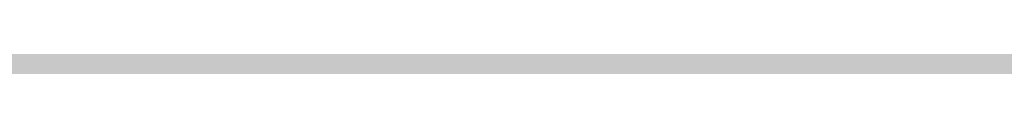
# Model space of a CAD drawing. Units: inches. Extents: x 2091 to 2899, y 967 to 2217.
# Tile 182 of 256: x 2203.16122 to 2203.18039, y 1152.24716 to 1152.24727. Entities that reach past the tile are written whole.
import ezdxf

# ---------------------------------------------------------------- set-up
doc = ezdxf.new("R2010")
doc.units = ezdxf.units.IN
doc.layers.add('A-WALL-PATT', color=141, linetype='Continuous', lineweight=13, true_color=0xadddf7)

msp = doc.modelspace()

# ---------------------------------------------------------------- hatches: boundary and pattern name
at = {"layer": 'A-WALL-PATT'}
h = msp.add_hatch(color=256, dxfattribs=at)
h.dxf.hatch_style = 1
h.paths.add_polyline_path([(2803.143603, 2050.919059), (2203.143603, 2050.919059), (2203.143603, 1090.919059), (2803.143603, 1090.919059)])
h.paths.add_polyline_path([(2635.79885, 1147.540465), (2674.524052, 1147.540465, 0.376086), (2678.529665, 1152.880202), (2678.529665, 1159.556473, 0.333335), (2674.524319, 1163.561846), (2674.524319, 1163.56185), (2674.524319, 1192.93439), (2635.805971, 1192.93439), (2597.087622, 1192.93439), (2597.087622, 1163.561846, 0.333335), (2593.082276, 1159.556473), (2593.082276, 1152.880202, 0.376086), (2597.087889, 1147.540465)], flags=0)
h.paths.add_polyline_path([(2436.010433, 1278.240778, 0.000483), (2435.952643, 1278.215027, -0.001328), (2435.935625, 1278.111693, -0.001711), (2436.11644, 1278.040758, 0.002185)], flags=0)
h.paths.add_polyline_path([(2794.143603, 1143.419059), (2794.143603, 1347.419059), (2543.370171, 1347.419059), (2543.370171, 1351.919059), (2794.143603, 1351.919059), (2794.143603, 1392.713555), (2793.947398, 1392.713555), (2793.947398, 1473.5369), (2794.143603, 1473.5369), (2794.143603, 1531.919059), (2650.143603, 1531.919059), (2650.143603, 1536.419059), (2794.143603, 1536.419059), (2794.143603, 1692.419059), (2609.375609, 1692.419059), (2609.375609, 1644.419059), (2604.875609, 1644.419059), (2604.875609, 1744.919059), (2609.375609, 1744.919059), (2609.375609, 1696.919059), (2794.143603, 1696.919059), (2794.143603, 1780.919059), (2609.643603, 1780.919059), (2493.875609, 1780.919059), (2493.875609, 1785.419059), (2609.643603, 1785.419059), (2794.143603, 1785.419059), (2794.143603, 1847.938821), (2793.951222, 1847.938821), (2793.951222, 1928.762166), (2794.143603, 1928.762166), (2794.143603, 1941.419059), (2614.143603, 1941.419059), (2614.143603, 1821.419059), (2609.643603, 1821.419059), (2609.643603, 1941.419059), (2392.143603, 1941.419059), (2392.143603, 1819.919059), (2387.643603, 1819.919059), (2387.643603, 1941.419059), (2212.143603, 1941.419059), (2212.143603, 1783.919059), (2392.143603, 1783.919059), (2392.143603, 1780.919059), (2212.143603, 1780.919059), (2212.143603, 1629.419059), (2387.643603, 1629.419059), (2387.643603, 1744.919059), (2392.143603, 1744.919059), (2392.143603, 1627.919059), (2317.143603, 1627.919059), (2317.143603, 1551.419059), (2317.143603, 1536.419059), (2459.383591, 1536.419059), (2459.383591, 1602.39648), (2463.883591, 1602.39648), (2463.883591, 1531.919059), (2456.643603, 1531.919059), (2456.643603, 1529.919059), (2452.143603, 1529.919059), (2452.143603, 1531.919059), (2312.643603, 1531.919059), (2312.643603, 1551.419059), (2306.143603, 1551.419059), (2306.143603, 1555.919059), (2308.143603, 1555.919059), (2308.143603, 1551.419059), (2312.643603, 1551.419059), (2312.643603, 1627.919059), (2212.143603, 1627.919059), (2212.143603, 1555.919059), (2270.143603, 1555.919059), (2270.143603, 1551.419059), (2212.143603, 1551.419059), (2212.143603, 1351.919059), (2272.143603, 1351.919059), (2272.143603, 1347.419059), (2212.143603, 1347.419059), (2212.143603, 1275.419059), (2308.143603, 1275.419059), (2308.143603, 1351.919059), (2452.143603, 1351.919059), (2452.143603, 1493.919059), (2456.643603, 1493.919059), (2456.643603, 1347.419059), (2312.643603, 1347.419059), (2312.643603, 1270.919059), (2212.143603, 1270.919059), (2212.143603, 1099.919059), (2281.237523, 1099.919059), (2282.871041, 1110.913803), (2282.008341, 1116.996603), (2278.557741, 1121.420403), (2268.205641, 1128.056203), (2272.087641, 1128.056203), (2273.812941, 1131.927003), (2279.420341, 1134.691903), (2285.027841, 1135.244903), (2287.615841, 1137.456803), (2288.047141, 1138.009803), (2289.341141, 1140.774703), (2291.066541, 1139.668703), (2292.360541, 1135.244903), (2295.379841, 1136.903803), (2296.242541, 1135.797903), (2297.105241, 1133.033003), (2300.124641, 1138.009803), (2303.143941, 1138.009803), (2304.437941, 1135.797903), (2303.143941, 1133.586003), (2306.594641, 1134.691903), (2307.888741, 1133.033003), (2310.908041, 1135.244903), (2313.927441, 1134.138903), (2315.62686, 1132.427102), (2308.320041, 1117.549603), (2290.203841, 1109.807903), (2288.909841, 1103.172103), (2289.272309, 1099.919059), (2434.918227, 1099.919059), (2431.593227, 1124.788059), (2429.930227, 1169.553059), (2430.927185, 1240.519694), (2435.658926, 1238.186126), (2437.135227, 1196.554059), (2438.798227, 1143.973059), (2442.678227, 1111.998059), (2446.558227, 1099.919059), (2794.143603, 1099.919059), (2794.143603, 1138.919059), (2548.032447, 1138.919059), (2548.032447, 1143.419059), (2548.032447, 1148.819059), (2546.668457, 1148.031559), (2528.685692, 1179.178622, 0.256256), (2512.032447, 1148.819059), (2512.032447, 1143.419059), (2512.032447, 1138.919059), (2507.532447, 1138.919059), (2507.532447, 1143.419059), (2507.532447, 1148.819059, 0.256256), (2490.879202, 1179.178622), (2472.896437, 1148.031559), (2471.532447, 1148.819059), (2471.532447, 1143.419059), (2467.032447, 1143.419059), (2467.032447, 1269.945786, 0.039061), (2460.909987, 1273.580059), (2467.032447, 1273.580059), (2467.032447, 1286.325364, 0.014511), (2465.216194, 1286.761905), (2467.032447, 1287.052576), (2467.032447, 1323.419059), (2471.532447, 1323.419059), (2471.532447, 1148.819059), (2489.532447, 1179.995973), (2490.896437, 1179.208473), (2490.879202, 1179.178622, -0.256256), (2507.532447, 1148.819059), (2507.532447, 1143.419059), (2512.032447, 1143.419059), (2512.032447, 1148.819059, -0.256256), (2528.685692, 1179.178622), (2528.668457, 1179.208473), (2530.032447, 1179.995973), (2548.032447, 1148.819059), (2548.032447, 1143.419059)], flags=16)
h.paths.add_polyline_path([(2607.768546, 1200.945083), (2607.768546, 1265.030625), (2597.087622, 1281.052011), (2619.784585, 1281.052011), (2627.795278, 1337.12686), (2635.79885, 1337.12686), (2643.816663, 1337.12686), (2651.827356, 1281.052011), (2674.524319, 1281.052011), (2663.843395, 1265.030625), (2663.843395, 1200.945083), (2635.805971, 1200.945083)], flags=0)
edge = h.paths.add_edge_path(flags=0)
edge.add_ellipse((13303.896215, 1272.998725), major_axis=(-10595.31304, 0.000001), ratio=0.842303870086, start_angle=0.6282372191, end_angle=0.6465540999, ccw=False)
edge.add_ellipse((2711.70045, 1156.852678), major_axis=(2.219769, 0), ratio=0.84230387, start_angle=111.535244, end_angle=180.628237, ccw=False)
edge.add_ellipse((13303.156292, 1272.998725), major_axis=(-10593.026306, 0), ratio=0.842303869544, start_angle=0.5282714718, end_angle=0.6465540971, ccw=False)
edge.add_line((2710.764596, 1175.333295), (2710.129986, 1175.333295))
edge.add_ellipse((2710.129986, 1176.579775), major_axis=(1.479846, 0), ratio=0.84230387, start_angle=180, end_angle=270, ccw=False)
edge.add_line((2708.65014, 1176.579775), (2708.65014, 1200.782914))
edge.add_ellipse((2710.129986, 1200.782914), major_axis=(1.479846, 0), ratio=0.84230387, start_angle=90, end_angle=180, ccw=False)
edge.add_line((2710.129986, 1202.029394), (2710.465075, 1202.029394))
edge.add_ellipse((13303.156292, 1272.998725), major_axis=(-10593.026306, 0), ratio=0.842303869544, start_angle=-0.0902290886, end_angle=0.3838667788, ccw=False)
edge.add_ellipse((2710.129986, 1290.927031), major_axis=(-1.479846, 0), ratio=0.84230387, start_angle=0, end_angle=90, ccw=False)
edge.add_line((2708.65014, 1290.927031), (2708.65014, 1315.13017))
edge.add_ellipse((2710.129986, 1315.13017), major_axis=(-1.479846, 0), ratio=0.84230387, start_angle=-90, end_angle=0, ccw=False)
edge.add_line((2710.129986, 1316.37665), (2710.706314, 1316.37665))
edge.add_ellipse((3238.40172, 1296.289566), major_axis=(528.234, 0), ratio=0.8423038695, start_angle=176.34957241, end_angle=177.82004969, ccw=False)
edge.add_ellipse((2775.063043, 1071.450696), major_axis=(313.307761, 0), ratio=0.8423038695, start_angle=102.12596555, end_angle=103.78052899, ccw=False)
edge.add_ellipse((2775.063043, 1078.305698), major_axis=(-305.302891, 0), ratio=0.8423038695, start_angle=-79.790461, end_angle=-77.55537271, ccw=False)
edge.add_ellipse((2695.141767, 1541.975383), major_axis=(-250.960216, 0), ratio=0.8423038695, start_angle=99.25656601, end_angle=102.55493264)
edge.add_line((2741.410326, 1334.214255), (2747.132545, 1337.378477))
edge.add_ellipse((2747.538616, 1336.857478), major_axis=(-0.739923, 0), ratio=0.8423039, start_angle=270, end_angle=307.93313, ccw=False)
edge.add_ellipse((2747.538616, 1336.857478), major_axis=(-0.739923, 0), ratio=0.8423039, start_angle=232.06687, end_angle=270, ccw=False)
edge.add_line((2747.944687, 1337.378477), (2753.666906, 1334.214255))
edge.add_ellipse((2799.935466, 1541.975383), major_axis=(250.960216, 0), ratio=0.8423038695, start_angle=257.44506736, end_angle=260.74343399)
edge.add_ellipse((2720.014189, 1078.305698), major_axis=(305.302891, 0), ratio=0.8423038695, start_angle=77.55537271, end_angle=79.790461, ccw=False)
edge.add_ellipse((2720.014189, 1071.450696), major_axis=(-313.307761, 0), ratio=0.8423038695, start_angle=256.21947101, end_angle=257.87403445, ccw=False)
edge.add_ellipse((2256.675512, 1296.289566), major_axis=(-528.234, 0), ratio=0.8423038695, start_angle=182.17995031, end_angle=183.65042759, ccw=False)
edge.add_line((2784.370918, 1316.37665), (2784.947247, 1316.37665))
edge.add_ellipse((2784.947247, 1315.13017), major_axis=(1.479846, 0), ratio=0.84230387, start_angle=0, end_angle=90, ccw=False)
edge.add_line((2786.427093, 1315.13017), (2786.427093, 1290.927031))
edge.add_ellipse((2784.947247, 1290.927031), major_axis=(1.479846, 0), ratio=0.84230387, start_angle=270, end_angle=360, ccw=False)
edge.add_ellipse((-7808.07906, 1272.998725), major_axis=(10593.026306, 0), ratio=0.842303869544, start_angle=-0.3838667788, end_angle=0.0902290886, ccw=False)
edge.add_line((2784.612157, 1202.029394), (2784.947247, 1202.029394))
edge.add_ellipse((2784.947247, 1200.782914), major_axis=(1.479846, 0), ratio=0.84230387, start_angle=0, end_angle=90, ccw=False)
edge.add_line((2786.427093, 1200.782914), (2786.427093, 1176.579775))
edge.add_ellipse((2784.947247, 1176.579775), major_axis=(-1.479846, 0), ratio=0.84230387, start_angle=90, end_angle=180, ccw=False)
edge.add_line((2784.947247, 1175.333295), (2784.312636, 1175.333295))
edge.add_ellipse((-7808.07906, 1272.998725), major_axis=(10593.026306, 0), ratio=0.842303869544, start_angle=-0.6186431963, end_angle=-0.5282714718, ccw=False)
edge.add_ellipse((2783.376783, 1156.852678), major_axis=(-2.219769, 0), ratio=0.84230387, start_angle=179.371763, end_angle=248.464757, ccw=False)
edge.add_ellipse((-7808.818983, 1272.998725), major_axis=(-10595.31304, 0.000004), ratio=0.842303865762, start_angle=179.3534459226, end_angle=179.3717628034, ccw=False)
edge.add_ellipse((2780.297303, 1153.500793), major_axis=(-5.246426, 0), ratio=0.84230387, start_angle=90, end_angle=179.353446, ccw=False)
edge.add_line((2780.297303, 1149.081708), (2714.77993, 1149.081708))
edge.add_ellipse((2714.77993, 1153.500793), major_axis=(5.246426, 0), ratio=0.84230387, start_angle=180.646554, end_angle=270, ccw=False)
edge = h.paths.add_edge_path(flags=0)
edge.add_line((2718.187367, 1151.007833), (2718.187367, 1170.472364))
edge.add_ellipse((2721.14706, 1170.472364), major_axis=(-2.959692, 0), ratio=0.84230387, start_angle=-90, end_angle=0, ccw=False)
edge.add_line((2721.14706, 1172.965324), (2773.930173, 1172.965324))
edge.add_ellipse((2773.930173, 1170.472364), major_axis=(-2.959692, 0), ratio=0.84230387, start_angle=180, end_angle=270, ccw=False)
edge.add_line((2776.889865, 1170.472364), (2776.889865, 1151.007833))
edge.add_line((2776.889865, 1151.007833), (2718.187367, 1151.007833))
edge = h.paths.add_edge_path(flags=0)
edge.add_line((2718.187367, 1180.23415), (2718.187367, 1199.057834))
edge.add_ellipse((2747.538616, 1320.39864), major_axis=(147.017924, 0), ratio=0.8423038695, start_angle=256.40186531, end_angle=283.59813469)
edge.add_line((2776.889865, 1199.057834), (2776.889865, 1180.23415))
edge.add_ellipse((2747.538616, 1301.574956), major_axis=(147.017924, 0), ratio=0.8423038695, start_angle=256.40186531, end_angle=283.59813469, ccw=False)
edge = h.paths.add_edge_path(flags=0)
edge.add_ellipse((13303.156292, 1272.998725), major_axis=(-10591.54646, 0), ratio=0.842303869555, start_angle=0.0555943135, end_angle=0.3777641939, ccw=False)
edge.add_line((2711.616859, 1262.72171), (2715.667408, 1249.495396))
edge.add_ellipse((6413.891963, 1241.691919), major_axis=(-3698.236159, 0), ratio=0.84230386955, start_angle=-0.120897369, end_angle=0.364076349)
edge.add_line((2715.761038, 1218.192455), (2711.934307, 1203.167361))
edge = h.paths.add_edge_path(flags=0)
edge.add_line((2718.187367, 1251.074566), (2716.002485, 1267.450435))
edge.add_ellipse((2742.151175, 1202.18954), major_axis=(81.772585, 0), ratio=0.84230387, start_angle=94.27742096, end_angle=111.8349538, ccw=False)
edge.add_line((2737.009748, 1270.930626), (2758.067484, 1270.930626))
edge.add_ellipse((2752.926058, 1202.18954), major_axis=(81.772585, 0), ratio=0.84230387, start_angle=68.1650462, end_angle=85.72257904, ccw=False)
edge.add_line((2779.074747, 1267.450435), (2776.889865, 1251.074566))
edge.add_ellipse((2750.338059, 1187.885356), major_axis=(79.579664, 0), ratio=0.84230387, start_angle=67.20808512, end_angle=85.1299304)
edge.add_line((2756.034656, 1254.743656), (2739.042576, 1254.743656))
edge.add_ellipse((2744.739174, 1187.885356), major_axis=(79.579664, 0), ratio=0.84230387, start_angle=94.8700696, end_angle=112.79191488)
edge = h.paths.add_edge_path(flags=0)
edge.add_line((2783.142926, 1203.167361), (2779.316194, 1218.192455))
edge.add_ellipse((-918.81473, 1241.691919), major_axis=(3698.236159, 0), ratio=0.84230386955, start_angle=-0.364076349, end_angle=0.120897369)
edge.add_line((2779.409825, 1249.495396), (2783.460373, 1262.72171))
edge.add_ellipse((-7808.07906, 1272.998725), major_axis=(-10591.54646, 0), ratio=0.84230386954, start_angle=179.6222358061, end_angle=179.9444056865, ccw=False)
edge = h.paths.add_edge_path(flags=0)
edge.add_ellipse((2734.200892, 1286.69044), major_axis=(-0.356609, 6.340078), ratio=0.60383358, start_angle=89.0020143, end_angle=253.657408, ccw=False)
edge.add_line((2730.369001, 1286.541806), (2730.369001, 1301.35198))
edge.add_line((2730.369001, 1301.35198), (2735.913311, 1305.214803))
edge.add_ellipse((2736.384917, 1304.734561), major_axis=(0.739923, 0), ratio=0.8423039, start_angle=90, end_angle=134.480211, ccw=False)
edge.add_line((2736.384917, 1305.357801), (2738.032783, 1305.357801))
edge.add_line((2738.032783, 1305.357801), (2738.032783, 1307.707927))
edge.add_ellipse((2794.201642, 1307.707927), major_axis=(56.168859, 0), ratio=0.84230387, start_angle=150.5614304, end_angle=180, ccw=False)
edge.add_ellipse((2700.875591, 1307.707927), major_axis=(-56.168859, 0), ratio=0.84230387, start_angle=180, end_angle=209.4385696, ccw=False)
edge.add_line((2757.04445, 1307.707927), (2757.04445, 1305.357801))
edge.add_line((2757.04445, 1305.357801), (2758.692316, 1305.357801))
edge.add_ellipse((2758.692316, 1304.734561), major_axis=(-0.739923, 0), ratio=0.8423039, start_angle=225.519789, end_angle=270, ccw=False)
edge.add_line((2759.163922, 1305.214803), (2764.708231, 1301.35198))
edge.add_line((2764.708231, 1301.35198), (2764.708231, 1286.541806))
edge.add_ellipse((2760.87634, 1286.69044), major_axis=(0.356609, 6.340078), ratio=0.60383358, start_angle=106.342592, end_angle=270.9979857, ccw=False)
edge.add_line((2757.04445, 1285.79709), (2757.04445, 1307.707927))
edge.add_ellipse((2700.875591, 1307.707927), major_axis=(-56.168859, 0), ratio=0.84230387, start_angle=180, end_angle=209.4385696)
edge.add_ellipse((2794.201642, 1307.707927), major_axis=(56.168859, 0), ratio=0.84230387, start_angle=150.5614304, end_angle=180)
edge.add_line((2738.032783, 1307.707927), (2738.032783, 1285.79709))
h.paths.add_polyline_path([(2417.812273, 1104.449704), (2413.492273, 1102.529704), (2410.612273, 1103.969704), (2409.172273, 1106.369704), (2407.252273, 1107.329704), (2406.292273, 1109.729704), (2405.332273, 1114.049704), (2405.332273, 1117.889704), (2406.292273, 1120.129704), (2407.252273, 1119.809704), (2408.848322, 1118.327658), (2410.173945, 1119.42417), (2410.211273, 1120.405704), (2411.040731, 1121.419054), (2410.699273, 1119.858704), (2410.173945, 1119.42417), (2410.088452, 1117.176109), (2411.132836, 1116.206324), (2413.972273, 1119.329704), (2416.852273, 1120.769704), (2416.869721, 1120.798784), (2417.035071, 1119.405116), (2417.896213, 1118.143384), (2418.292273, 1118.369704), (2419.544447, 1120.039269), (2419.360915, 1118.387487), (2419.032108, 1119.356151), (2418.398939, 1118.511926), (2419.252273, 1114.529704), (2418.794091, 1107.198795)], flags=0)
h.paths.add_polyline_path([(2508.870171, 1347.419059), (2508.370171, 1347.419059), (2508.370171, 1351.919059), (2508.870171, 1351.919059)], flags=0)
h.paths.add_polyline_path([(2473.370171, 1347.419059), (2472.370171, 1347.419059), (2467.870171, 1347.419059), (2467.870171, 1455.419059), (2472.370171, 1455.419059), (2472.370171, 1352.419059), (2473.370171, 1352.419059)], flags=0)
h.paths.add_polyline_path([(2352.106244, 1217.446197), (2349.226244, 1218.886197), (2347.786244, 1221.286197), (2345.866244, 1222.246197), (2344.906244, 1224.646197), (2343.946244, 1228.966197), (2343.946244, 1232.806197), (2344.906244, 1235.046197), (2345.866244, 1234.726197), (2347.462293, 1233.244152), (2348.787916, 1234.340663), (2348.825244, 1235.322197), (2349.654702, 1236.335547), (2349.313244, 1234.775197), (2348.787916, 1234.340663), (2348.702423, 1232.092603), (2349.746807, 1231.122817), (2352.586244, 1234.246197), (2355.466244, 1235.686197), (2355.483692, 1235.715277), (2355.649043, 1234.321609), (2356.510185, 1233.059877), (2356.906244, 1233.286197), (2358.158418, 1234.955762), (2357.974887, 1233.30398), (2357.646079, 1234.272644), (2357.012911, 1233.428419), (2357.866244, 1229.446197), (2357.408062, 1222.115288), (2356.426244, 1219.366197)], flags=0)
h.paths.add_polyline_path([(2348.2968, 1112.22442), (2347.0138, 1112.31042), (2345.5298, 1114.12742), (2345.7318, 1115.85842), (2346.8118, 1116.98242), (2346.8118, 1114.64642), (2345.8668, 1114.21442), (2346.8798, 1114.30042)], flags=0)
h.paths.add_polyline_path([(2347.0138, 1110.92642), (2346.2718, 1110.49342), (2346.6098, 1111.18642)], flags=0)
h.paths.add_polyline_path([(2345.8668, 1118.19442), (2345.5298, 1117.32942), (2343.7078, 1118.02142), (2344.3828, 1118.62642)], flags=0)
h.paths.add_polyline_path([(2346.6768, 1109.28242), (2346.0698, 1108.07142), (2345.8668, 1110.06142)], flags=0)
h.paths.add_polyline_path([(2345.0568, 1119.75142), (2343.6398, 1119.75142), (2343.9778, 1121.13542)], flags=0)
h.paths.add_polyline_path([(2345.2598, 1116.55042), (2345.1248, 1115.85842), (2344.9218, 1115.68542), (2344.7198, 1116.37742)], flags=0)
h.paths.add_polyline_path([(2345.6648, 1112.31042), (2345.4618, 1111.53242), (2344.0448, 1111.96442), (2344.6518, 1112.57042)], flags=0)
h.paths.add_polyline_path([(2345.1918, 1113.34942), (2344.4498, 1113.86842), (2344.7198, 1114.38742)], flags=0)
h.paths.add_polyline_path([(2344.6518, 1116.80942), (2344.1798, 1115.68542), (2344.6518, 1115.33942), (2343.9098, 1114.90642), (2343.0328, 1115.94442), (2343.6398, 1116.46342)], flags=0)
h.paths.add_polyline_path([(2345.8668, 1106.68642), (2344.9898, 1105.56242), (2344.5168, 1106.60042)], flags=0)
h.paths.add_polyline_path([(2344.8548, 1110.06142), (2344.5168, 1109.28242), (2344.1128, 1109.71542)], flags=0)
h.paths.add_polyline_path([(2344.0448, 1113.52242), (2343.4378, 1113.08942), (2342.7628, 1113.95442)], flags=0)
h.paths.add_polyline_path([(2344.3148, 1111.01242), (2342.9648, 1110.32042), (2342.9648, 1111.09942)], flags=0)
h.paths.add_polyline_path([(2345.1248, 1104.69742), (2344.5848, 1103.74542), (2344.4498, 1104.26442)], flags=0)
h.paths.add_polyline_path([(2342.8298, 1121.22242), (2341.7498, 1120.53042), (2340.5358, 1121.04942), (2340.1308, 1121.82842), (2340.6708, 1122.95242), (2341.1428, 1121.82842), (2341.6148, 1122.00142)], flags=0)
h.paths.add_polyline_path([(2342.9648, 1119.75142), (2343.0328, 1118.45342), (2342.0878, 1118.02142), (2342.0198, 1119.49142)], flags=0)
h.paths.add_polyline_path([(2342.6948, 1116.89642), (2341.9528, 1116.63642), (2342.0198, 1117.32942)], flags=0)
h.paths.add_polyline_path([(2343.0328, 1112.22442), (2342.0198, 1111.79142), (2341.5478, 1112.22442), (2342.3578, 1113.34942)], flags=0)
h.paths.add_polyline_path([(2343.7748, 1104.43742), (2342.6278, 1102.88042), (2342.6948, 1104.61042), (2343.4378, 1105.12942)], flags=0)
h.paths.add_polyline_path([(2342.0198, 1115.07942), (2340.8058, 1115.51242), (2340.9408, 1116.37742)], flags=0)
h.paths.add_polyline_path([(2341.4808, 1120.09742), (2341.4808, 1119.40542), (2341.0758, 1119.57842), (2341.1428, 1120.09742)], flags=0)
h.paths.add_polyline_path([(2341.8178, 1114.47342), (2340.9408, 1113.08942), (2340.8058, 1114.56042)], flags=0)
h.paths.add_polyline_path([(2341.1428, 1118.54042), (2340.9408, 1116.98242), (2339.0508, 1117.67542), (2339.0508, 1118.62642)], flags=0)
h.paths.add_polyline_path([(2342.6948, 1101.66842), (2341.9528, 1101.84142), (2342.5598, 1102.36142)], flags=0)
h.paths.add_polyline_path([(2340.3328, 1119.66542), (2338.4438, 1119.57842), (2337.9038, 1120.35742), (2339.6578, 1120.61642)], flags=0)
h.paths.add_polyline_path([(2340.3328, 1115.33942), (2340.0628, 1113.69542), (2339.3878, 1115.33942)], flags=0)
h.paths.add_polyline_path([(2341.8178, 1103.83142), (2341.5478, 1102.88042), (2341.1428, 1103.65842)], flags=0)
h.paths.add_polyline_path([(2339.0508, 1122.86642), (2337.2958, 1121.82842), (2337.0938, 1123.12542), (2337.7688, 1123.81842)], flags=0)
h.paths.add_polyline_path([(2339.1178, 1121.74142), (2338.8478, 1121.22242), (2338.1738, 1121.04942), (2338.3758, 1121.56842)], flags=0)
h.paths.add_polyline_path([(2339.1858, 1119.31942), (2338.6458, 1118.71342), (2338.2408, 1118.10742), (2338.2408, 1118.88642)], flags=0)
h.paths.add_polyline_path([(2341.1428, 1101.92842), (2340.6028, 1101.23642), (2340.0628, 1101.84142), (2340.6028, 1102.36142)], flags=0)
h.paths.add_polyline_path([(2337.6338, 1117.76142), (2336.6208, 1118.28042), (2337.2958, 1118.97242)], flags=0)
h.paths.add_polyline_path([(2336.8238, 1119.57842), (2334.7988, 1118.97242), (2335.2038, 1120.35742), (2336.5538, 1120.87642)], flags=0)
h.paths.add_polyline_path([(2339.1178, 1100.45742), (2337.3638, 1100.54342), (2336.7558, 1101.23642)], flags=0)
h.paths.add_polyline_path([(2336.3508, 1122.43342), (2336.0138, 1121.91442), (2334.9338, 1122.43342), (2334.5288, 1123.47142), (2335.7438, 1122.77942)], flags=0)
h.paths.add_polyline_path([(2334.7318, 1120.87642), (2334.2588, 1120.35742), (2334.0568, 1120.78942), (2334.5968, 1121.30842)], flags=0)
h.paths.add_polyline_path([(2334.4618, 1122.17442), (2332.5718, 1121.30842), (2331.3568, 1122.17442), (2332.0998, 1122.86642)], flags=0)
h.paths.add_polyline_path([(2334.2588, 1118.54042), (2333.3818, 1118.45342), (2333.6518, 1119.31942)], flags=0)
h.paths.add_polyline_path([(2335.5418, 1102.27442), (2334.1918, 1102.62042), (2335.2718, 1103.31242)], flags=0)
h.paths.add_polyline_path([(2332.7068, 1119.66542), (2331.6948, 1120.44342), (2332.5048, 1120.78942)], flags=0)
h.paths.add_polyline_path([(2334.7318, 1101.14942), (2333.5168, 1101.58242), (2333.9888, 1101.75542)], flags=0)
h.paths.add_polyline_path([(2332.6398, 1116.63642), (2331.0868, 1116.29042), (2331.9648, 1118.19442)], flags=0)
h.paths.add_polyline_path([(2330.7498, 1121.56842), (2330.2768, 1120.27042), (2328.5228, 1119.31942), (2328.9948, 1121.04942)], flags=0)
h.paths.add_polyline_path([(2330.7498, 1118.62642), (2330.0078, 1117.50242), (2329.8728, 1118.02142)], flags=0)
h.paths.add_polyline_path([(2332.0998, 1102.36142), (2330.5468, 1102.01442), (2331.6948, 1102.96642)], flags=0)
h.paths.add_polyline_path([(2329.5348, 1113.60842), (2329.0628, 1112.31042), (2328.5898, 1113.34942)], flags=0)
h.paths.add_polyline_path([(2328.3878, 1117.84842), (2327.5098, 1116.55042), (2327.1728, 1117.76142)], flags=0)
h.paths.add_polyline_path([(2329.7378, 1106.51342), (2329.5348, 1105.30242), (2328.2528, 1106.08142)], flags=0)
h.paths.add_polyline_path([(2328.6578, 1114.38742), (2328.0498, 1114.12742), (2328.3198, 1114.90642)], flags=0)
h.paths.add_polyline_path([(2328.3198, 1112.22442), (2327.1058, 1112.13742), (2326.7008, 1112.65642)], flags=0)
h.paths.add_polyline_path([(2326.9028, 1115.25242), (2326.7008, 1114.12742), (2325.2158, 1113.60842), (2326.0928, 1115.33942)], flags=0)
h.paths.add_polyline_path([(2326.6328, 1108.33042), (2326.0928, 1107.37942), (2325.8908, 1108.50342), (2326.4978, 1109.10942)], flags=0)
h.paths.add_polyline_path([(2615.143603, 1531.919059), (2609.643603, 1531.919059), (2609.643603, 1620.419059), (2614.143603, 1620.419059), (2614.143603, 1536.419059), (2615.143603, 1536.419059)], flags=0)
h.paths.add_polyline_path([(2545.143603, 1563.419059), (2464.143603, 1563.419059), (2464.143603, 1632.419059), (2509.143603, 1632.419059), (2509.143603, 1627.919059), (2509.143603, 1603.919059), (2468.643603, 1603.919059), (2468.643603, 1567.919059), (2540.643603, 1567.919059), (2540.643603, 1591.919059), (2545.143603, 1591.919059)], flags=0)
h.paths.add_polyline_path([(2388.969048, 1549.985735), (2357.434181, 1549.985735), (2357.434181, 1623.360778), (2399.362777, 1623.360778), (2435.689465, 1623.360778), (2435.592547, 1602.559273), (2435.592547, 1602.39648), (2388.969048, 1602.39648)], flags=0)
h.paths.add_polyline_path([(2388.880628, 1555.809151), (2374.904429, 1555.809151), (2374.904429, 1600.571564), (2374.904429, 1615.457645), (2406.350877, 1615.457645), (2406.350877, 1618.939431), (2412.174293, 1615.457645), (2406.350877, 1611.97586), (2406.350877, 1615.457645), (2388.880628, 1615.457645)], flags=0)
h.paths.add_polyline_path([(2568.875609, 1644.419059), (2453.375609, 1644.419059), (2453.375609, 1785.419059), (2457.875609, 1785.419059), (2457.875609, 1648.919059), (2568.875609, 1648.919059)], flags=0)
h.paths.add_polyline_path([(2212.143603, 1945.919059), (2212.143603, 2041.919059), (2794.143603, 2041.919059), (2794.143603, 1945.919059)], flags=16)
h.paths.add_polyline_path([(2271.082728, 1964.317238), (2776.852968, 1964.317238), (2776.852968, 2037.169623), (2271.082728, 2037.169623)], flags=8)
h.paths.add_polyline_path([(2380.649285, 1536.824144), (2461.040809, 1536.824144), (2461.040809, 1554.652587), (2380.649285, 1554.652587)], flags=8)
h.paths.add_polyline_path([(2240.755709, 1609.725451), (2309.185829, 1609.725451), (2309.185829, 1617.698204), (2240.755709, 1617.698204)], flags=8)
h.paths.add_polyline_path([(2212.677255, 1313.504102), (2282.59152, 1313.504102), (2282.59152, 1322.745239), (2212.677255, 1322.745239)], flags=8)
h.paths.add_polyline_path([(2457.111976, 1114.778574), (2558.481581, 1114.778574), (2558.481581, 1142.219682), (2457.111976, 1142.219682)], flags=8)
h.paths.add_polyline_path([(2473.442337, 1273.010067), (2604.641226, 1273.010067), (2604.641226, 1318.346935), (2473.442337, 1318.346935)], flags=8)
h.paths.add_polyline_path([(2638.876302, 1626.977432), (2684.250367, 1627.976738), (2684.038483, 1637.597494), (2638.664417, 1636.598188)], flags=8)
h.paths.add_polyline_path([(2537.590554, 1453.793447), (2628.389547, 1453.793447), (2628.389547, 1475.344811), (2537.590554, 1475.344811)], flags=8)
h.paths.add_polyline_path([(2504.137638, 1714.632397), (2554.647187, 1714.632397), (2554.647187, 1730.237712), (2504.137638, 1730.237712)], flags=8)
h.paths.add_polyline_path([(2487.501181, 1575.651872), (2535.097121, 1575.651872), (2535.097121, 1598.377646), (2487.501181, 1598.377646)], flags=8)
h.paths.add_polyline_path([(2709.0994, 1735.710278), (2740.016601, 1735.710278), (2740.016601, 1749.937641), (2709.0994, 1749.937641)], flags=8)
h.paths.add_polyline_path([(2442.438424, 1792.171657), (2564.728835, 1792.171657), (2564.728835, 1842.000163), (2442.438424, 1842.000163)], flags=8)
h.paths.add_polyline_path([(2655.815801, 1809.644076), (2789.520142, 1806.693796), (2790.084977, 1832.291638), (2656.380635, 1835.241918)], flags=8)
h.paths.add_polyline_path([(2234.842697, 1797.720143), (2368.592851, 1794.768852), (2369.160718, 1820.504132), (2235.410564, 1823.455423)], flags=8)
h.paths.add_polyline_path([(2245.138466, 1644.006335), (2398.427733, 1640.6239), (2398.994842, 1666.32482), (2245.705575, 1669.707255)], flags=8)
h.paths.add_polyline_path([(2306.142847, 1431.168519), (2413.768314, 1428.793687), (2414.333148, 1454.391529), (2306.707682, 1456.76636)], flags=8)
h.paths.add_polyline_path([(2306.834582, 1458.233145), (2393.380484, 1456.323449), (2393.932808, 1481.354358), (2307.386907, 1483.264054)], flags=8)

doc.saveas('drawing.dxf')
